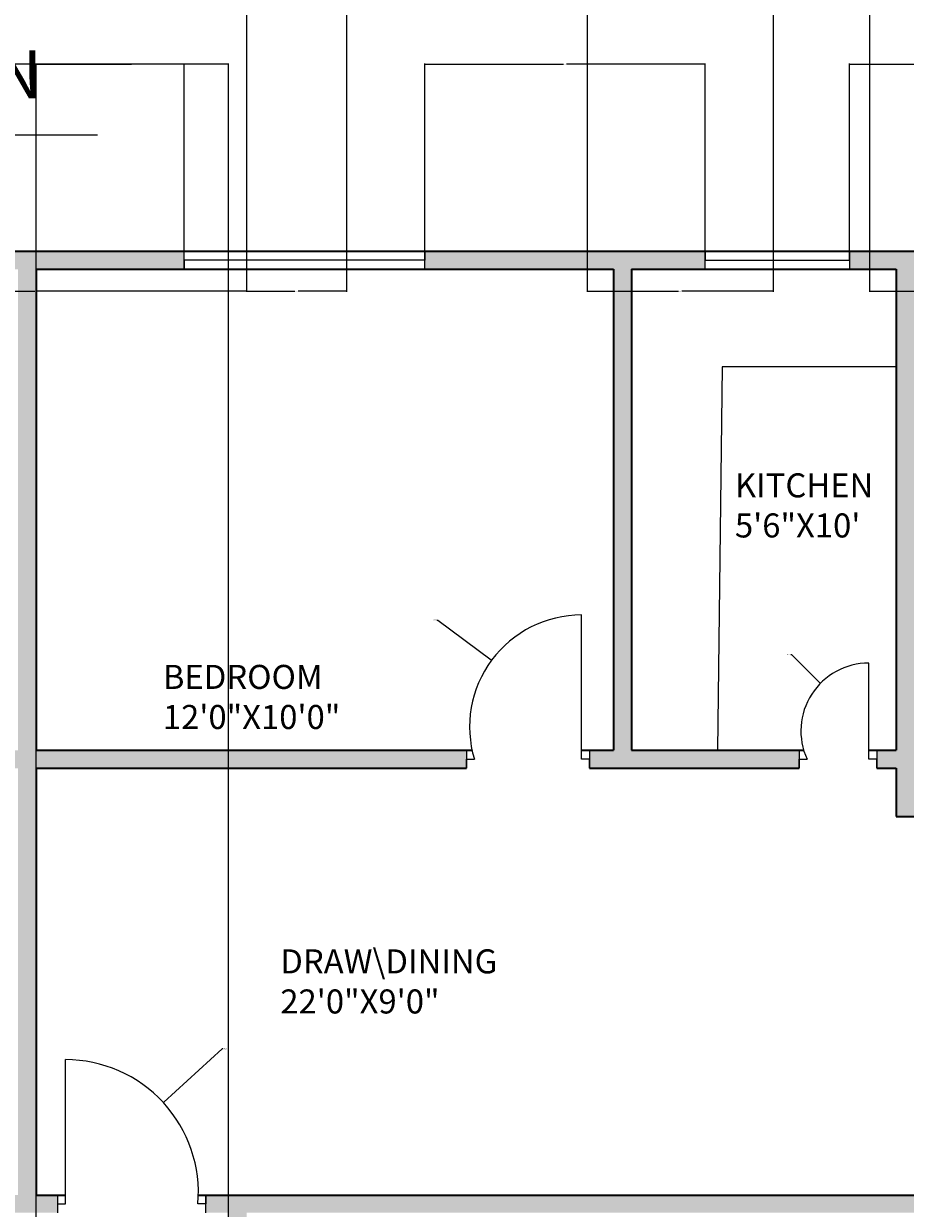
# Model space of a CAD drawing. Units: inches. Extents: x 2314 to 3223, y 1382 to 2735.
# Tile 12 of 14: x 2767 to 2987, y 2143 to 2439. Entities that reach past the tile are written whole.
import ezdxf

# ---------------------------------------------------------------- set-up
doc = ezdxf.new("R2010")
doc.units = ezdxf.units.IN
for name, color, linetype, lineweight in [('A-ANNO-DIMS', 2, 'Continuous', 18), ('A-ANNO-TEXT', 7, 'Continuous', 25), ('A-AREA-IDEN', 7, 'Continuous', 18), ('A-DOOR', 3, 'Continuous', 18), ('A-FLOR-FIXT', 8, 'Continuous', 18), ('A-GLAZ', 4, 'Continuous', 18), ('A-WALL', 7, 'Continuous', 35)]:
    doc.layers.add(name, color=color, linetype=linetype, lineweight=lineweight)
doc.layers.add('A-WALL-PATT', color=251, linetype='Continuous', lineweight=13, true_color=0x636466)
doc.styles.get("Standard").update_dxf_attribs({"font": 'arial.ttf'})
doc.dimstyles.get("Standard").update_dxf_attribs({"dimtxt": 0.18, "dimasz": 0.18, "dimexe": 0.18, "dimexo": 0.0625, "dimgap": 0.09, "dimtad": 0, "dimtih": 1, "dimtoh": 1, "dimdec": 4, "dimzin": 0, "dimdsep": 46, "dimtxsty": 'Standard', "dimcen": 0.09, "dimadec": 0, "dimazin": 0, "dimtfac": 1, "dimtdec": 4, "dimtofl": 0, "dimtmove": 0, "dimatfit": 3, "dimfxl": 1, "dimtolj": 1, "dimtzin": 0, "dimarcsym": 0})

# ---------------------------------------------------------------- blocks, each defined once
blk = doc.blocks.new('WIN-PLAN-60')
for p, q in [((0, 4.5), (0, 0)), ((60, 2.25), (60, 4.5)), ((60, 4.5), (60, 0)), ((0, 0), (0, 2.25)), ((0, 2.25), (60, 2.25))]:
    blk.add_line(p, q)
blk = doc.blocks.new('WIN-PLAN-36-ALT')
for p, q in [((0, 36), (4.5, 36)), ((4.5, 36), (2.25, 36)), ((2.25, 36), (2.25, 0)), ((4.5, 0), (0, 0)), ((2.25, 0), (4.5, 0))]:
    blk.add_line(p, q)
blk = doc.blocks.new('*D30')
at = {"layer": 'A-ANNO-DIMS', "color": 0, "lineweight": -2, "transparency": 16777216}
for p, q in [((3125.96, 2381.78), (3172.77, 2381.78)), ((3172.59, 2381.6), (3172.59, 1973.38)), ((3172.59, 1564.8), (3172.59, 1973.02)), ((2822.96, 1564.62), (3172.77, 1564.62))]:
    blk.add_line(p, q, dxfattribs=at)
at = {"layer": 'A-ANNO-DIMS', "color": 0, "transparency": 16777216}
for points in [[(3172.56, 2381.6), (3172.62, 2381.6), (3172.59, 2381.78)], [(3172.56, 1564.8), (3172.62, 1564.8), (3172.59, 1564.62)]]:
    blk.add_solid(points, dxfattribs=at)
at = {"layer": 'Defpoints', "color": 0, "transparency": 16777216}
for p in [(3125.89, 2381.78), (2822.89, 1564.62), (3172.59, 1564.62)]:
    blk.add_point(p, dxfattribs=at)
at = {"layer": 'A-ANNO-DIMS', "color": 0, "transparency": 16777216, "insert": (3172.59, 1973.2), "char_height": 0.18, "attachment_point": 5}
blk.add_mtext('\\A1;817.2', dxfattribs=at)
blk = doc.blocks.new('*D39')
at = {"layer": 'A-ANNO-DIMS', "color": 0, "lineweight": -2, "transparency": 16777216}
for p, q in [((2770.39, 1744.06), (2770.39, 2428.66)), ((2770.57, 2428.48), (2794.17, 2428.48)), ((2818.21, 2428.48), (2794.62, 2428.48)), ((2818.39, 1744.06), (2818.39, 2428.66))]:
    blk.add_line(p, q, dxfattribs=at)
at = {"layer": 'A-ANNO-DIMS', "color": 0, "transparency": 16777216}
for points in [[(2770.57, 2428.51), (2770.57, 2428.45), (2770.39, 2428.48)], [(2818.21, 2428.51), (2818.21, 2428.45), (2818.39, 2428.48)]]:
    blk.add_solid(points, dxfattribs=at)
at = {"layer": 'Defpoints', "color": 0, "transparency": 16777216}
for p in [(2818.39, 2428.48), (2770.39, 1744), (2818.39, 1744)]:
    blk.add_point(p, dxfattribs=at)
at = {"layer": 'A-ANNO-DIMS', "color": 0, "transparency": 16777216, "insert": (2794.39, 2428.48), "char_height": 0.18, "attachment_point": 5}
blk.add_mtext('\\A1;48', dxfattribs=at)
blk = doc.blocks.new('*D43')
at = {"layer": 'A-ANNO-DIMS', "color": 0, "lineweight": -2, "transparency": 16777216}
for p, q in [((2716.06, 2381.85), (2716.06, 2428.66)), ((2716.24, 2428.48), (2761.31, 2428.48)), ((2807.16, 2428.48), (2762.1, 2428.48)), ((2807.34, 2381.85), (2807.34, 2428.66))]:
    blk.add_line(p, q, dxfattribs=at)
at = {"layer": 'A-ANNO-DIMS', "color": 0, "transparency": 16777216}
for points in [[(2716.24, 2428.51), (2716.24, 2428.45), (2716.06, 2428.48)], [(2807.16, 2428.51), (2807.16, 2428.45), (2807.34, 2428.48)]]:
    blk.add_solid(points, dxfattribs=at)
at = {"layer": 'Defpoints', "color": 0, "transparency": 16777216}
for p in [(2807.34, 2428.48), (2716.06, 2381.78), (2807.34, 2381.78)]:
    blk.add_point(p, dxfattribs=at)
at = {"layer": 'A-ANNO-DIMS', "color": 0, "transparency": 16777216, "insert": (2761.7, 2428.48), "char_height": 0.18, "attachment_point": 5}
blk.add_mtext('\\A1;91.28', dxfattribs=at)
blk = doc.blocks.new('*D44')
at = {"layer": 'A-ANNO-DIMS', "color": 0, "lineweight": -2, "transparency": 16777216}
for p, q in [((2867.34, 2381.85), (2867.34, 2428.66)), ((2867.52, 2428.48), (2901.88, 2428.48)), ((2937.03, 2428.48), (2902.67, 2428.48)), ((2937.21, 2381.85), (2937.21, 2428.66))]:
    blk.add_line(p, q, dxfattribs=at)
at = {"layer": 'A-ANNO-DIMS', "color": 0, "transparency": 16777216}
for points in [[(2867.52, 2428.51), (2867.52, 2428.45), (2867.34, 2428.48)], [(2937.03, 2428.51), (2937.03, 2428.45), (2937.21, 2428.48)]]:
    blk.add_solid(points, dxfattribs=at)
at = {"layer": 'Defpoints', "color": 0, "transparency": 16777216}
for p in [(2937.21, 2428.48), (2867.34, 2381.78), (2937.21, 2381.78)]:
    blk.add_point(p, dxfattribs=at)
at = {"layer": 'A-ANNO-DIMS', "color": 0, "transparency": 16777216, "insert": (2902.28, 2428.48), "char_height": 0.18, "attachment_point": 5}
blk.add_mtext('\\A1;69.87', dxfattribs=at)
blk = doc.blocks.new('*D45')
at = {"layer": 'A-ANNO-DIMS', "color": 0, "lineweight": -2, "transparency": 16777216}
for p, q in [((2973.21, 2381.85), (2973.21, 2428.66)), ((2973.39, 2428.48), (2997.29, 2428.48)), ((3021.98, 2428.48), (2998.08, 2428.48)), ((3022.16, 2381.85), (3022.16, 2428.66))]:
    blk.add_line(p, q, dxfattribs=at)
at = {"layer": 'A-ANNO-DIMS', "color": 0, "transparency": 16777216}
for points in [[(2973.39, 2428.51), (2973.39, 2428.45), (2973.21, 2428.48)], [(3021.98, 2428.51), (3021.98, 2428.45), (3022.16, 2428.48)]]:
    blk.add_solid(points, dxfattribs=at)
at = {"layer": 'Defpoints', "color": 0, "transparency": 16777216}
for p in [(3022.16, 2428.48), (2973.21, 2381.78), (3022.16, 2381.78)]:
    blk.add_point(p, dxfattribs=at)
at = {"layer": 'A-ANNO-DIMS', "color": 0, "transparency": 16777216, "insert": (2997.69, 2428.48), "char_height": 0.18, "attachment_point": 5}
blk.add_mtext('\\A1;48.95', dxfattribs=at)
blk = doc.blocks.new('*D56')
at = {"layer": 'A-ANNO-DIMS', "color": 0, "lineweight": -2, "transparency": 16777216}
for p, q in [((2717.89, 2466.62), (2717.89, 2371.63)), ((2822.89, 2466.62), (2822.89, 2371.63)), ((2718.07, 2371.81), (2770.11, 2371.81)), ((2822.71, 2371.81), (2770.67, 2371.81))]:
    blk.add_line(p, q, dxfattribs=at)
at = {"layer": 'A-ANNO-DIMS', "color": 0, "transparency": 16777216}
for points in [[(2718.07, 2371.84), (2718.07, 2371.78), (2717.89, 2371.81)], [(2822.71, 2371.84), (2822.71, 2371.78), (2822.89, 2371.81)]]:
    blk.add_solid(points, dxfattribs=at)
at = {"layer": 'Defpoints', "color": 0, "transparency": 16777216}
for p in [(2717.89, 2466.68), (2822.89, 2466.68), (2822.89, 2371.81)]:
    blk.add_point(p, dxfattribs=at)
at = {"layer": 'A-ANNO-DIMS', "color": 0, "transparency": 16777216, "insert": (2770.39, 2371.81), "char_height": 0.18, "attachment_point": 5}
blk.add_mtext('\\A1;105', dxfattribs=at)
blk = doc.blocks.new('*D57')
at = {"layer": 'A-ANNO-DIMS', "color": 0, "lineweight": -2, "transparency": 16777216}
for p, q in [((2847.78, 2502.62), (2847.78, 2371.63)), ((2822.89, 2466.62), (2822.89, 2371.63)), ((2823.07, 2371.81), (2834.94, 2371.81)), ((2847.6, 2371.81), (2835.73, 2371.81))]:
    blk.add_line(p, q, dxfattribs=at)
at = {"layer": 'A-ANNO-DIMS', "color": 0, "transparency": 16777216}
for points in [[(2823.07, 2371.84), (2823.07, 2371.78), (2822.89, 2371.81)], [(2847.6, 2371.84), (2847.6, 2371.78), (2847.78, 2371.81)]]:
    blk.add_solid(points, dxfattribs=at)
at = {"layer": 'Defpoints', "color": 0, "transparency": 16777216}
for p in [(2847.78, 2502.68), (2822.89, 2466.68), (2847.78, 2371.81)]:
    blk.add_point(p, dxfattribs=at)
at = {"layer": 'A-ANNO-DIMS', "color": 0, "transparency": 16777216, "insert": (2835.34, 2371.81), "char_height": 0.18, "attachment_point": 5}
blk.add_mtext('\\A1;24.89', dxfattribs=at)
blk = doc.blocks.new('*D58')
at = {"layer": 'A-ANNO-DIMS', "color": 0, "lineweight": -2, "transparency": 16777216}
for p, q in [((2907.78, 2502.62), (2907.78, 2371.63)), ((2954.22, 2502.62), (2954.22, 2371.63)), ((2907.96, 2371.81), (2930.61, 2371.81)), ((2954.04, 2371.81), (2931.4, 2371.81))]:
    blk.add_line(p, q, dxfattribs=at)
at = {"layer": 'A-ANNO-DIMS', "color": 0, "transparency": 16777216}
for points in [[(2907.96, 2371.84), (2907.96, 2371.78), (2907.78, 2371.81)], [(2954.04, 2371.84), (2954.04, 2371.78), (2954.22, 2371.81)]]:
    blk.add_solid(points, dxfattribs=at)
at = {"layer": 'Defpoints', "color": 0, "transparency": 16777216}
for p in [(2907.78, 2502.68), (2954.22, 2502.68), (2954.22, 2371.81)]:
    blk.add_point(p, dxfattribs=at)
at = {"layer": 'A-ANNO-DIMS', "color": 0, "transparency": 16777216, "insert": (2931, 2371.81), "char_height": 0.18, "attachment_point": 5}
blk.add_mtext('\\A1;46.44', dxfattribs=at)
blk = doc.blocks.new('*D59')
at = {"layer": 'A-ANNO-DIMS', "color": 0, "lineweight": -2, "transparency": 16777216}
for p, q in [((2978.22, 2502.62), (2978.22, 2371.63)), ((3034.7, 2502.62), (3034.7, 2371.63)), ((2978.4, 2371.81), (3006.07, 2371.81)), ((3034.52, 2371.81), (3006.85, 2371.81))]:
    blk.add_line(p, q, dxfattribs=at)
at = {"layer": 'A-ANNO-DIMS', "color": 0, "transparency": 16777216}
for points in [[(2978.4, 2371.84), (2978.4, 2371.78), (2978.22, 2371.81)], [(3034.52, 2371.84), (3034.52, 2371.78), (3034.7, 2371.81)]]:
    blk.add_solid(points, dxfattribs=at)
at = {"layer": 'Defpoints', "color": 0, "transparency": 16777216}
for p in [(2978.22, 2502.68), (3034.7, 2502.68), (3034.7, 2371.81)]:
    blk.add_point(p, dxfattribs=at)
at = {"layer": 'A-ANNO-DIMS', "color": 0, "transparency": 16777216, "insert": (3006.46, 2371.81), "char_height": 0.18, "attachment_point": 5}
blk.add_mtext('\\A1;56.47', dxfattribs=at)
blk = doc.blocks.new('*D64')
at = {"layer": 'A-ANNO-DIMS', "color": 0, "lineweight": -2, "transparency": 16777216}
for p, q in [((2816.79, 2182.78), (2802.27, 2169.46)), ((2816.97, 2182.78), (2816.79, 2182.78)), ((2777.62, 2146.94), (2777.8, 2146.94)), ((2777.71, 2146.85), (2777.71, 2147.03))]:
    blk.add_line(p, q, dxfattribs=at)
at = {"layer": 'A-ANNO-DIMS', "color": 0, "transparency": 16777216}
blk.add_solid([(2802.25, 2169.49), (2802.29, 2169.44), (2802.14, 2169.34)], dxfattribs=at)
at = {"layer": 'Defpoints', "color": 0, "transparency": 16777216}
for p in [(2802.14, 2169.34), (2777.71, 2146.94)]:
    blk.add_point(p, dxfattribs=at)
at = {"layer": 'A-ANNO-DIMS', "color": 0, "transparency": 16777216, "insert": (2817.45, 2182.78), "char_height": 0.18, "attachment_point": 5}
blk.add_mtext('\\A1;R33.14', dxfattribs=at)
blk = doc.blocks.new('*D75')
at = {"layer": 'A-ANNO-DIMS', "color": 0, "lineweight": -2, "transparency": 16777216}
for p, q in [((2870.36, 2289.74), (2870.54, 2289.74)), ((2870.54, 2289.74), (2883.85, 2279.86)), ((2906.32, 2263.11), (2906.5, 2263.11)), ((2906.41, 2263.02), (2906.41, 2263.2))]:
    blk.add_line(p, q, dxfattribs=at)
at = {"layer": 'A-ANNO-DIMS', "color": 0, "transparency": 16777216}
blk.add_solid([(2883.87, 2279.89), (2883.83, 2279.84), (2883.99, 2279.76)], dxfattribs=at)
at = {"layer": 'Defpoints', "color": 0, "transparency": 16777216}
for p in [(2883.99, 2279.76), (2906.41, 2263.11)]:
    blk.add_point(p, dxfattribs=at)
at = {"layer": 'A-ANNO-DIMS', "color": 0, "transparency": 16777216, "insert": (2869.88, 2289.74), "char_height": 0.18, "attachment_point": 5}
blk.add_mtext('\\A1;R27.92', dxfattribs=at)
blk = doc.blocks.new('*D90')
at = {"layer": 'A-ANNO-DIMS', "color": 0, "lineweight": -2, "transparency": 16777216}
for p, q in [((2958.59, 2281.15), (2958.77, 2281.15)), ((2958.77, 2281.15), (2965.87, 2274.12)), ((2977.97, 2262.08), (2978.15, 2262.08)), ((2978.06, 2261.99), (2978.06, 2262.17))]:
    blk.add_line(p, q, dxfattribs=at)
at = {"layer": 'A-ANNO-DIMS', "color": 0, "transparency": 16777216}
blk.add_solid([(2965.9, 2274.15), (2965.85, 2274.1), (2966, 2274)], dxfattribs=at)
at = {"layer": 'Defpoints', "color": 0, "transparency": 16777216}
for p in [(2966, 2274), (2978.06, 2262.08)]:
    blk.add_point(p, dxfattribs=at)
at = {"layer": 'A-ANNO-DIMS', "color": 0, "transparency": 16777216, "insert": (2958.11, 2281.15), "char_height": 0.18, "attachment_point": 5}
blk.add_mtext('\\A1;R16.95', dxfattribs=at)

msp = doc.modelspace()

# ---------------------------------------------------------------- hatches: boundary and pattern name
at = {"layer": 'A-WALL-PATT'}
h = msp.add_hatch(color=256, dxfattribs=at)
h.dxf.hatch_style = 1
h.paths.add_polyline_path([(2443.3302, 2379.5332), (2443.3302, 2381.7832), (2410.3927, 2381.7832), (2410.3927, 2336.7008), (2414.8927, 2336.7008), (2414.8927, 2377.2832), (2443.3302, 2377.2832)])
h.paths.add_polyline_path([(2561.3645, 2379.5332), (2561.3645, 2381.7832), (2503.3302, 2381.7832), (2503.3302, 2377.2832), (2546.8927, 2377.2832), (2546.8927, 2245.2832), (2541.8787, 2245.2832), (2541.8787, 2240.7832), (2551.3927, 2240.7832), (2551.3927, 2377.2832), (2561.3645, 2377.2832)])
h.paths.add_polyline_path([(2656.0607, 2381.7832), (2597.3645, 2381.7832), (2597.3645, 2377.2832), (2617.3927, 2377.2832), (2617.3927, 2257.2832), (2584.2532, 2257.2832), (2584.2532, 2252.7832), (2625.8528, 2252.7832), (2625.8528, 2255.0332), (2625.8528, 2257.2832), (2621.8927, 2257.2832), (2621.8927, 2377.2832), (2656.0607, 2377.2832), (2656.0607, 2379.5332)])
h.paths.add_polyline_path([(2807.3418, 2381.7832), (2716.0607, 2381.7832), (2716.0607, 2377.2832), (2765.8927, 2377.2832), (2765.8927, 2257.2832), (2661.6935, 2257.2832), (2661.6935, 2252.7832), (2765.8927, 2252.7832), (2765.8927, 2146.2832), (2760.9259, 2146.2832), (2760.9259, 2141.8832), (2775.7119, 2141.8832), (2775.7119, 2146.2832), (2770.3927, 2146.2832), (2770.3927, 2252.7832), (2877.684, 2252.7832), (2877.684, 2255.0332), (2877.684, 2257.2832), (2770.3927, 2257.2832), (2770.3927, 2377.2832), (2807.3418, 2377.2832), (2807.3418, 2379.5332)])
h.paths.add_polyline_path([(2937.2118, 2381.7832), (2867.3418, 2381.7832), (2867.3418, 2377.2832), (2914.3927, 2377.2832), (2914.3927, 2257.2832), (2908.4124, 2257.2832), (2908.4124, 2252.7832), (2960.6432, 2252.7832), (2960.6432, 2255.0332), (2960.6432, 2257.2832), (2918.8927, 2257.2832), (2918.8927, 2377.2832), (2937.2118, 2377.2832)])
h.paths.add_polyline_path([(3022.1601, 2381.7832), (2973.2118, 2381.7832), (2973.2118, 2379.5332), (2973.2118, 2377.2832), (2984.8927, 2377.2832), (2984.8927, 2257.2832), (2980.0601, 2257.2832), (2980.0601, 2252.7832), (2984.8927, 2252.7832), (2984.8927, 2240.7832), (2995.668, 2240.7832), (2995.668, 2243.0332), (2995.668, 2245.2832), (2989.3927, 2245.2832), (2989.3927, 2377.2832), (3022.1601, 2377.2832), (3022.1601, 2379.5332)])
h.paths.add_polyline_path([(3125.8927, 2381.7832), (3082.1601, 2381.7832), (3082.1601, 2377.2832), (3121.3927, 2377.2832), (3121.3927, 2334.7388), (3125.8927, 2334.7388)])
h.paths.add_polyline_path([(3125.8927, 2274.7388), (3121.3927, 2274.7388), (3121.3927, 2245.2832), (3066.4832, 2245.2832), (3066.4832, 2240.7832), (3121.3927, 2240.7832), (3121.3927, 2232.1868), (3125.8927, 2232.1868)])
h.paths.add_polyline_path([(3125.8927, 2208.1868), (3121.3927, 2208.1868), (3121.3927, 2198.7832), (3037.3927, 2198.7832), (3037.3927, 2240.7832), (3041.2694, 2240.7832), (3041.2694, 2243.0332), (3041.2694, 2245.2832), (3026.8205, 2245.2832), (3026.8205, 2240.7832), (3032.8927, 2240.7832), (3032.8927, 2190.4022), (3037.3927, 2190.4022), (3037.3927, 2194.2832), (3121.3927, 2194.2832), (3121.3927, 2182.1835), (3125.8927, 2182.1835)])
h.paths.add_polyline_path([(3125.8927, 2158.1835), (3121.3927, 2158.1835), (3121.3927, 2146.2832), (3037.3927, 2146.2832), (3037.3927, 2169.3726), (3035.1427, 2169.3726), (3032.8927, 2169.3726), (3032.8927, 2146.2832), (2812.7301, 2146.2832), (2812.7301, 2144.0832), (2812.7301, 2141.8832), (2818.3927, 2141.8832), (2818.3927, 1970.1316), (2822.8927, 1970.1316), (2822.8927, 1978.8832), (2903.9846, 1978.8832), (2903.9846, 1981.1332), (2903.9846, 1983.3832), (2822.8927, 1983.3832), (2822.8927, 2115.3832), (2851.7162, 2115.3832), (2851.7162, 2117.6332), (2851.7162, 2119.8832), (2822.8927, 2119.8832), (2822.8927, 2141.8832), (3125.8927, 2141.8832)])
h.paths.add_polyline_path([(3125.8927, 2119.8832), (3081.193, 2119.8832), (3081.193, 2115.3832), (3121.3927, 2115.3832), (3121.3927, 2071.8188), (3125.8927, 2071.8188)], flags=17)
h.paths.add_polyline_path([(2989.3927, 2115.3832), (3021.193, 2115.3832), (3021.193, 2117.6332), (3021.193, 2119.8832), (2979.123, 2119.8832), (2979.123, 2115.3832), (2984.8927, 2115.3832), (2984.8927, 2019.3832), (2981.9225, 2019.3832), (2981.9225, 2014.8832), (2984.8927, 2014.8832), (2984.8927, 1983.3832), (2984.8927, 1978.8832), (2989.3927, 1978.8832), (2989.3927, 1983.3832)], flags=17)
h.paths.add_polyline_path([(2947.3927, 2115.3832), (2955.123, 2115.3832), (2955.123, 2117.6332), (2955.123, 2119.8832), (2911.7162, 2119.8832), (2911.7162, 2115.3832), (2942.8927, 2115.3832), (2942.8927, 1983.3832), (2936.7017, 1983.3832), (2936.7017, 1978.8832), (2947.3927, 1978.8832), (2947.3927, 1983.3832), (2947.3927, 2014.8832), (2960.7167, 2014.8832), (2960.7167, 2017.1332), (2960.7167, 2019.3832), (2947.3927, 2019.3832)], flags=17)
h.paths.add_polyline_path([(3037.3927, 1978.8832), (3041.8276, 1978.8832), (3041.8276, 1981.1332), (3041.8276, 1983.3832), (3025.477, 1983.3832), (3025.477, 1978.8832), (3032.8927, 1978.8832), (3032.8927, 1927.1259), (3035.1427, 1927.1259), (3037.3927, 1927.1259)])
h.paths.add_polyline_path([(3125.8927, 2011.8188), (3123.6427, 2011.8188), (3121.3927, 2011.8188), (3121.3927, 1983.3832), (3065, 1983.3832), (3065, 1978.8832), (3121.3927, 1978.8832), (3121.3927, 1970.5932), (3125.8927, 1970.5932)], flags=17)
h.paths.add_polyline_path([(2994.2341, 1983.3832), (2989.3927, 1983.3832), (2989.3927, 1978.8832), (2994.2341, 1978.8832), (2994.2341, 1981.1332)], flags=16)
h.paths.add_polyline_path([(3125.8927, 1946.5932), (3121.3927, 1946.5932), (3121.3927, 1936.8832), (3037.3927, 1936.8832), (3037.3927, 1932.3832), (3121.3927, 1932.3832), (3121.3927, 1919.825), (3125.8927, 1919.825)])
h.paths.add_polyline_path([(3125.8927, 1883.825), (3121.3927, 1883.825), (3121.3927, 1866.3832), (3037.3927, 1866.3832), (3037.3927, 1899.0954), (3035.1427, 1899.0954), (3032.8927, 1899.0954), (3032.8927, 1866.3832), (2822.8927, 1866.3832), (2822.8927, 1938.7212), (2820.6427, 1938.7212), (2818.3927, 1938.7212), (2818.3927, 1786.9239), (2822.8927, 1786.9239), (2822.8927, 1861.8832), (3032.8927, 1861.8832), (3032.8927, 1825.1023), (3037.3927, 1825.1023), (3037.3927, 1861.8832), (3121.3927, 1861.8832), (3121.3927, 1844.6765), (3125.8927, 1844.6765)])
h.paths.add_polyline_path([(3125.8927, 1808.6765), (3121.3927, 1808.6765), (3121.3927, 1795.8832), (3037.3927, 1795.8832), (3037.3927, 1799.4755), (3032.8927, 1799.4755), (3032.8927, 1749.3832), (3026.5034, 1749.3832), (3026.5034, 1744.8832), (3032.8927, 1744.8832), (3034.9255, 1744.8832), (3043.1326, 1744.8832), (3043.1326, 1747.1332), (3043.1326, 1749.3832), (3037.3927, 1749.3832), (3037.3927, 1791.3832), (3121.3927, 1791.3832), (3121.3927, 1783.3103), (3125.8927, 1783.3103)])
h.paths.add_polyline_path([(3125.8927, 1759.3103), (3121.3927, 1759.3103), (3121.3927, 1749.3832), (3065.1845, 1749.3832), (3065.1845, 1744.8832), (3121.3927, 1744.8832), (3121.3927, 1709.3573), (3125.8927, 1709.3573)])
h.paths.add_polyline_path([(3125.8927, 1649.3573), (3121.3927, 1649.3573), (3121.3927, 1612.8832), (3095.116, 1612.8832), (3095.116, 1608.3832), (3125.8927, 1608.3832)])
h.paths.add_polyline_path([(3035.116, 1612.8832), (2993.8927, 1612.8832), (2993.8927, 1744.8832), (2998.7409, 1744.8832), (2998.7409, 1749.3832), (2989.3927, 1749.3832), (2989.3927, 1744.8832), (2989.3927, 1701.3832), (2972.8226, 1701.3832), (2972.8226, 1696.8832), (2989.3927, 1696.8832), (2989.3927, 1612.8832), (2978.2225, 1612.8832), (2978.2225, 1608.3832), (3035.116, 1608.3832), (3035.116, 1610.6332)])
h.paths.add_polyline_path([(2947.3927, 1696.8832), (2950.7566, 1696.8832), (2950.7566, 1699.1332), (2950.7566, 1701.3832), (2947.3927, 1701.3832), (2947.3927, 1744.8832), (2947.3927, 1749.3832), (2937.649, 1749.3832), (2937.649, 1744.8832), (2942.8927, 1744.8832), (2942.8927, 1612.8832), (2907.783, 1612.8832), (2907.783, 1608.3832), (2954.2225, 1608.3832), (2954.2225, 1610.6332), (2954.2225, 1612.8832), (2947.3927, 1612.8832)])
h.paths.add_polyline_path([(2822.8927, 1744.8832), (2905.3491, 1744.8832), (2905.3491, 1747.1332), (2905.3491, 1749.3832), (2822.8927, 1749.3832), (2822.8927, 1756.9185), (2818.3927, 1756.9185), (2818.3927, 1612.8832), (2818.3927, 1569.1205), (2722.3927, 1569.1205), (2722.3927, 1612.8832), (2722.3927, 1756.9185), (2717.8927, 1756.9185), (2717.8927, 1750.0143), (2633.6297, 1750.0143), (2633.6437, 1745.2665), (2717.8927, 1745.5143), (2717.8927, 1612.8832), (2689.8467, 1612.8832), (2689.8467, 1608.3832), (2717.8927, 1608.3832), (2717.8927, 1564.6205), (2722.3927, 1564.6205), (2822.8927, 1564.6205), (2822.8927, 1569.1205), (2822.8927, 1608.3832), (2847.783, 1608.3832), (2847.783, 1610.6332), (2847.783, 1612.8832), (2822.8927, 1612.8832)])
h.paths.add_polyline_path([(2629.8467, 1612.8832), (2597.8927, 1612.8832), (2597.8927, 1744.8832), (2597.8927, 1745.1613), (2601.5887, 1745.1721), (2601.5816, 1747.5932), (2601.5745, 1750.0143), (2593.3927, 1750.0143), (2593.3927, 1744.8832), (2593.3927, 1713.3832), (2589.7588, 1713.3832), (2589.7588, 1708.8832), (2593.3927, 1708.8832), (2593.3927, 1612.8832), (2582.3793, 1612.8832), (2582.3793, 1608.3832), (2629.8467, 1608.3832), (2629.8467, 1610.6332)])
h.paths.add_polyline_path([(2551.3927, 1708.8832), (2567.6776, 1708.8832), (2567.6776, 1711.1332), (2567.6776, 1713.3832), (2551.3927, 1713.3832), (2551.3927, 1744.8832), (2551.3927, 1750.0143), (2543.5657, 1750.0143), (2543.5657, 1747.5079), (2543.5657, 1745.0014), (2546.8927, 1745.0112), (2546.8927, 1744.8832), (2546.8927, 1612.8832), (2502.9339, 1612.8832), (2502.9339, 1608.3832), (2558.3793, 1608.3832), (2558.3793, 1610.6332), (2558.3793, 1612.8832), (2551.3927, 1612.8832)])
h.paths.add_polyline_path([(2414.8927, 1656.2547), (2410.3927, 1656.2547), (2410.3927, 1608.3832), (2442.9339, 1608.3832), (2442.9339, 1610.6332), (2442.9339, 1612.8832), (2414.8927, 1612.8832)])
h.paths.add_polyline_path([(2414.8927, 1744.8832), (2468.8906, 1744.8832), (2468.8906, 1747.1332), (2468.8906, 1749.3832), (2414.8927, 1749.3832), (2414.8927, 1757.7622), (2410.3927, 1757.7622), (2410.3927, 1716.2547), (2414.8927, 1716.2547)])
h.paths.add_polyline_path([(2414.8927, 1791.3832), (2498.8927, 1791.3832), (2498.8927, 1749.3832), (2492.9799, 1749.3832), (2492.9799, 1744.8832), (2498.8927, 1744.8832), (2503.3927, 1744.8832), (2508.0135, 1744.8968), (2508.0059, 1747.4556), (2507.9984, 1750.0143), (2503.3927, 1750.0143), (2503.3927, 1802.6362), (2501.1427, 1802.6362), (2498.8927, 1802.6362), (2498.8927, 1795.8832), (2414.8927, 1795.8832), (2414.8927, 1808.0943), (2410.3927, 1808.0943), (2410.3927, 1781.7622), (2414.8927, 1781.7622)])
h.paths.add_polyline_path([(2722.3927, 1937.589), (2720.1427, 1937.589), (2717.8927, 1937.589), (2717.8927, 1866.3832), (2503.3927, 1866.3832), (2503.3927, 1896.3484), (2498.8927, 1896.3484), (2498.8927, 1866.3832), (2414.8927, 1866.3832), (2414.8927, 1882.1496), (2410.3927, 1882.1496), (2410.3927, 1844.0943), (2414.8927, 1844.0943), (2414.8927, 1861.8832), (2498.8927, 1861.8832), (2498.8927, 1831.4783), (2501.1427, 1831.4783), (2503.3927, 1831.4783), (2503.3927, 1861.8832), (2717.8927, 1861.8832), (2717.8927, 1786.9239), (2722.3927, 1786.9239)])
h.paths.add_polyline_path([(2414.8927, 1932.3832), (2498.8927, 1932.3832), (2498.8927, 1924.7883), (2503.3927, 1924.7883), (2503.3927, 1978.8832), (2505.8599, 1978.8832), (2505.8599, 1981.1332), (2505.8599, 1983.3832), (2493.3697, 1983.3832), (2493.3697, 1978.8832), (2498.8927, 1978.8832), (2498.8927, 1936.8832), (2414.8927, 1936.8832), (2414.8927, 1943.2834), (2410.3927, 1943.2834), (2410.3927, 1918.1496), (2414.8927, 1918.1496)])
h.paths.add_polyline_path([(2414.8927, 2020.3133), (2412.6427, 2020.3133), (2410.3927, 2020.3133), (2410.3927, 1967.2834), (2414.8927, 1967.2834), (2414.8927, 1978.8832), (2468.8513, 1978.8832), (2468.8513, 1981.1332), (2468.8513, 1983.3832), (2414.8927, 1983.3832)])
h.paths.add_polyline_path([(2414.8927, 2115.3832), (2453.004, 2115.3832), (2453.004, 2117.6332), (2453.004, 2119.8832), (2410.3927, 2119.8832), (2410.3927, 2080.3133), (2414.8927, 2080.3133)], flags=17)
h.paths.add_polyline_path([(2559.0969, 2117.6332), (2559.0969, 2119.8832), (2513.004, 2119.8832), (2513.004, 2115.3832), (2546.8927, 2115.3832), (2546.8927, 1983.3832), (2542.7531, 1983.3832), (2542.7531, 1978.8832), (2551.3927, 1978.8832), (2551.3927, 2014.8832), (2570.3098, 2014.8832), (2570.3098, 2017.1332), (2570.3098, 2019.3832), (2551.3927, 2019.3832), (2551.3927, 2115.3832), (2559.0969, 2115.3832)], flags=17)
h.paths.add_polyline_path([(2628.5073, 2117.6332), (2628.5073, 2119.8832), (2583.0969, 2119.8832), (2583.0969, 2115.3832), (2593.3927, 2115.3832), (2593.3927, 2019.3832), (2590.2108, 2019.3832), (2590.2108, 2014.8832), (2593.3927, 2014.8832), (2593.3927, 1978.8832), (2601.5907, 1978.8832), (2601.5907, 1981.1332), (2601.5907, 1983.3832), (2597.8927, 1983.3832), (2597.8927, 2115.3832), (2628.5073, 2115.3832)], flags=17)
h.paths.add_polyline_path([(2722.3927, 2141.8832), (2726.9871, 2141.8832), (2726.9871, 2144.2705), (2726.9871, 2146.2832), (2503.3927, 2146.2832), (2503.3927, 2168.2161), (2501.1427, 2168.2161), (2498.8927, 2168.2161), (2498.8927, 2146.2832), (2414.8927, 2146.2832), (2414.8927, 2156.5041), (2410.3927, 2156.5041), (2410.3927, 2141.8832), (2717.8927, 2141.8832), (2717.8927, 2119.8832), (2688.5073, 2119.8832), (2688.5073, 2115.3832), (2717.8927, 2115.3832), (2717.8927, 1983.3832), (2633.2454, 1983.3832), (2633.2454, 1978.8832), (2717.8927, 1978.8832), (2717.8927, 1970.1316), (2720.1427, 1970.1316), (2722.3927, 1970.1316)])
h.paths.add_polyline_path([(2557.3704, 1462.9278), (2940.0934, 1462.9278), (2940.0934, 1512.3848), (2557.3704, 1512.3848)], flags=9)
h.paths.add_polyline_path([(2846.2527, 1703.1384), (2892.8612, 1703.1384), (2892.8612, 1725.5272), (2846.2527, 1725.5272)], flags=25)
h.paths.add_polyline_path([(2885.6102, 1812.1147), (2946.1505, 1812.1147), (2946.1505, 1834.5035), (2885.6102, 1834.5035)], flags=25)
h.paths.add_polyline_path([(2885.6102, 1884.183), (2946.1505, 1884.183), (2946.1505, 1906.5718), (2885.6102, 1906.5718)], flags=25)
h.paths.add_polyline_path([(3066.365, 1705.5431), (3112.9735, 1705.5431), (3112.9735, 1727.9319), (3066.365, 1727.9319)], flags=9)
h.paths.add_polyline_path([(3061.8255, 1887.7513), (3101.6154, 1887.7513), (3101.6154, 1910.1401), (3061.8255, 1910.1401)], flags=25)
h.paths.add_polyline_path([(3063.3679, 1816.2121), (3103.1578, 1816.2121), (3103.1578, 1838.6009), (3063.3679, 1838.6009)], flags=25)
h.paths.add_polyline_path([(3053.3743, 1768.416), (3107.1329, 1768.416), (3107.1329, 1790.8048), (3053.3743, 1790.8048)], flags=25)
h.paths.add_polyline_path([(3061.6068, 1943.822), (3115.3653, 1943.822), (3115.3653, 1966.2109), (3061.6068, 1966.2109)], flags=9)
h.paths.add_polyline_path([(2745.0978, 1763.6604), (2797.9354, 1763.6604), (2797.9354, 1776.0247), (2745.0978, 1776.0247)], flags=9)
h.paths.add_polyline_path([(2574.2135, 1819.2586), (2634.7538, 1819.2586), (2634.7538, 1841.6474), (2574.2135, 1841.6474)], flags=25)
h.paths.add_polyline_path([(2574.2135, 1891.3269), (2634.7538, 1891.3269), (2634.7538, 1913.7157), (2574.2135, 1913.7157)], flags=25)
h.paths.add_polyline_path([(2638.4466, 1702.43), (2685.0551, 1702.43), (2685.0551, 1724.8188), (2638.4466, 1724.8188)], flags=25)
h.paths.add_polyline_path([(2435.9715, 1697.1215), (2482.5799, 1697.1215), (2482.5799, 1719.5103), (2435.9715, 1719.5103)], flags=9)
h.paths.add_polyline_path([(2431.2046, 1893.7833), (2470.9945, 1893.7833), (2470.9945, 1916.1721), (2431.2046, 1916.1721)], flags=25)
h.paths.add_polyline_path([(2439.8144, 1817.2116), (2479.6043, 1817.2116), (2479.6043, 1839.6004), (2439.8144, 1839.6004)], flags=25)
h.paths.add_polyline_path([(2441.2607, 1753.0942), (2495.0192, 1753.0942), (2495.0192, 1775.483), (2441.2607, 1775.483)], flags=25)
h.paths.add_polyline_path([(2421.216, 1945.3109), (2474.9746, 1945.3109), (2474.9746, 1967.6997), (2421.216, 1967.6997)], flags=25)
h.paths.add_polyline_path([(2585.4464, 1627.5703), (2585.4464, 1679), (2563.0576, 1679), (2563.0576, 1627.5703)], flags=9)
h.paths.add_polyline_path([(2978.3497, 1618.7039), (2978.3497, 1670.1337), (2955.9609, 1670.1337), (2955.9609, 1618.7039)], flags=9)
h.paths.add_polyline_path([(2975.9502, 2041.7828), (2975.9502, 2093.2125), (2953.5614, 2093.2125), (2953.5614, 2041.7828)], flags=25)
h.paths.add_polyline_path([(2835.6537, 1989.2068), (2882.2621, 1989.2068), (2882.2621, 2011.5956), (2835.6537, 2011.5956)], flags=25)
h.paths.add_polyline_path([(2649.3769, 1997.5659), (2695.9853, 1997.5659), (2695.9853, 2019.9547), (2649.3769, 2019.9547)], flags=25)
h.paths.add_polyline_path([(2579.9087, 2040.3429), (2579.9087, 2091.7726), (2557.5198, 2091.7726), (2557.5198, 2040.3429)], flags=25)
h.paths.add_polyline_path([(2783.2404, 1883.1956), (2783.2404, 2067.1369), (2764.694, 2067.1369), (2764.694, 1883.1956)], flags=9)
h.paths.add_polyline_path([(3055.8435, 1993.5571), (3102.4519, 1993.5571), (3102.4519, 2015.9459), (3055.8435, 2015.9459)], flags=25)
h.paths.add_polyline_path([(2423.6009, 1984.6082), (2470.2094, 1984.6082), (2470.2094, 2006.997), (2423.6009, 2006.997)], flags=25)
h.paths.add_polyline_path([(2973.4115, 2123.1668), (3013.1319, 2123.1668), (3013.1319, 2135.531), (2973.4115, 2135.531)], flags=25)
h.paths.add_polyline_path([(2534.3846, 2124.6231), (2574.105, 2124.6231), (2574.105, 2136.9874), (2534.3846, 2136.9874)], flags=25)
h.paths.add_polyline_path([(2829.1368, 2188.1931), (2889.411, 2188.1931), (2889.411, 2210.5819), (2829.1368, 2210.5819)], flags=9)
h.paths.add_polyline_path([(2633.2547, 2185.0437), (2693.5289, 2185.0437), (2693.5289, 2207.4325), (2633.2547, 2207.4325)], flags=9)
h.paths.add_polyline_path([(2445.1812, 2167.0395), (2496.611, 2167.0395), (2496.611, 2189.4284), (2445.1812, 2189.4284)], flags=9)
h.paths.add_polyline_path([(2429.1678, 2194.5482), (2480.5975, 2194.5482), (2480.5975, 2216.937), (2429.1678, 2216.937)], flags=9)
h.paths.add_polyline_path([(3060.1138, 2158.1056), (3111.5436, 2158.1056), (3111.5436, 2180.4944), (3060.1138, 2180.4944)], flags=9)
h.paths.add_polyline_path([(3055.6824, 2201.2631), (3107.1122, 2201.2631), (3107.1122, 2223.652), (3055.6824, 2223.652)], flags=25)
h.paths.add_polyline_path([(3044.3482, 2257.7345), (3090.9567, 2257.7345), (3090.9567, 2280.1233), (3044.3482, 2280.1233)], flags=9)
h.paths.add_polyline_path([(2942.5437, 2306.9625), (2982.3336, 2306.9625), (2982.3336, 2329.3513), (2942.5437, 2329.3513)], flags=9)
h.paths.add_polyline_path([(2799.5865, 2259.1663), (2846.195, 2259.1663), (2846.195, 2281.5551), (2799.5865, 2281.5551)], flags=25)
h.paths.add_polyline_path([(2670.4998, 2261.1493), (2717.1082, 2261.1493), (2717.1082, 2283.5381), (2670.4998, 2283.5381)], flags=25)
h.paths.add_polyline_path([(2553.0333, 2302.7735), (2592.8232, 2302.7735), (2592.8232, 2325.1624), (2553.0333, 2325.1624)], flags=9)
h.paths.add_polyline_path([(2432.0288, 2268.6489), (2478.6372, 2268.6489), (2478.6372, 2291.0377), (2432.0288, 2291.0377)], flags=9)
h = msp.add_hatch(color=256, dxfattribs=at)
h.dxf.hatch_style = 1
h.paths.add_polyline_path([(2503.3927, 2240.7832), (2507.7952, 2240.7832), (2507.7952, 2245.2832), (2496.4262, 2245.2832), (2496.4262, 2243.0332), (2496.4262, 2240.7832), (2498.8927, 2240.7832), (2498.8927, 2198.7832), (2414.8927, 2198.7832), (2414.8927, 2206.5718), (2410.3927, 2206.5718), (2410.3927, 2180.5041), (2412.6427, 2180.5041), (2414.8927, 2180.5041), (2414.8927, 2194.2832), (2498.8927, 2194.2832), (2498.8927, 2191.0069), (2503.3927, 2191.0069)])
h.paths.add_polyline_path([(2414.8927, 2276.7008), (2410.3927, 2276.7008), (2410.3927, 2230.5718), (2414.8927, 2230.5718), (2414.8927, 2240.7832), (2474.2564, 2240.7832), (2474.2564, 2243.0332), (2474.2564, 2245.2832), (2414.8927, 2245.2832)])
h.paths.add_polyline_path([(2557.3704, 1462.9278), (2940.0934, 1462.9278), (2940.0934, 1512.3848), (2557.3704, 1512.3848)], flags=9)
h.paths.add_polyline_path([(2846.2527, 1703.1384), (2892.8612, 1703.1384), (2892.8612, 1725.5272), (2846.2527, 1725.5272)], flags=9)
h.paths.add_polyline_path([(2885.6102, 1812.1147), (2946.1505, 1812.1147), (2946.1505, 1834.5035), (2885.6102, 1834.5035)], flags=9)
h.paths.add_polyline_path([(2885.6102, 1884.183), (2946.1505, 1884.183), (2946.1505, 1906.5718), (2885.6102, 1906.5718)], flags=9)
h.paths.add_polyline_path([(3066.365, 1705.5431), (3112.9735, 1705.5431), (3112.9735, 1727.9319), (3066.365, 1727.9319)], flags=9)
h.paths.add_polyline_path([(3061.8255, 1887.7513), (3101.6154, 1887.7513), (3101.6154, 1910.1401), (3061.8255, 1910.1401)], flags=9)
h.paths.add_polyline_path([(3063.3679, 1816.2121), (3103.1578, 1816.2121), (3103.1578, 1838.6009), (3063.3679, 1838.6009)], flags=9)
h.paths.add_polyline_path([(3053.3743, 1768.416), (3107.1329, 1768.416), (3107.1329, 1790.8048), (3053.3743, 1790.8048)], flags=9)
h.paths.add_polyline_path([(3061.6068, 1943.822), (3115.3653, 1943.822), (3115.3653, 1966.2109), (3061.6068, 1966.2109)], flags=9)
h.paths.add_polyline_path([(2745.0978, 1763.6604), (2797.9354, 1763.6604), (2797.9354, 1776.0247), (2745.0978, 1776.0247)], flags=9)
h.paths.add_polyline_path([(2574.2135, 1819.2586), (2634.7538, 1819.2586), (2634.7538, 1841.6474), (2574.2135, 1841.6474)], flags=9)
h.paths.add_polyline_path([(2574.2135, 1891.3269), (2634.7538, 1891.3269), (2634.7538, 1913.7157), (2574.2135, 1913.7157)], flags=9)
h.paths.add_polyline_path([(2638.4466, 1702.43), (2685.0551, 1702.43), (2685.0551, 1724.8188), (2638.4466, 1724.8188)], flags=9)
h.paths.add_polyline_path([(2435.9715, 1697.1215), (2482.5799, 1697.1215), (2482.5799, 1719.5103), (2435.9715, 1719.5103)], flags=9)
h.paths.add_polyline_path([(2431.2046, 1893.7833), (2470.9945, 1893.7833), (2470.9945, 1916.1721), (2431.2046, 1916.1721)], flags=9)
h.paths.add_polyline_path([(2439.8144, 1817.2116), (2479.6043, 1817.2116), (2479.6043, 1839.6004), (2439.8144, 1839.6004)], flags=9)
h.paths.add_polyline_path([(2441.2607, 1753.0942), (2495.0192, 1753.0942), (2495.0192, 1775.483), (2441.2607, 1775.483)], flags=9)
h.paths.add_polyline_path([(2421.216, 1945.3109), (2474.9746, 1945.3109), (2474.9746, 1967.6997), (2421.216, 1967.6997)], flags=9)
h.paths.add_polyline_path([(2585.4464, 1627.5703), (2585.4464, 1679), (2563.0576, 1679), (2563.0576, 1627.5703)], flags=9)
h.paths.add_polyline_path([(2978.3497, 1618.7039), (2978.3497, 1670.1337), (2955.9609, 1670.1337), (2955.9609, 1618.7039)], flags=9)
h.paths.add_polyline_path([(2975.9502, 2041.7828), (2975.9502, 2093.2125), (2953.5614, 2093.2125), (2953.5614, 2041.7828)], flags=9)
h.paths.add_polyline_path([(2835.6537, 1989.2068), (2882.2621, 1989.2068), (2882.2621, 2011.5956), (2835.6537, 2011.5956)], flags=9)
h.paths.add_polyline_path([(2649.3769, 1997.5659), (2695.9853, 1997.5659), (2695.9853, 2019.9547), (2649.3769, 2019.9547)], flags=9)
h.paths.add_polyline_path([(2579.9087, 2040.3429), (2579.9087, 2091.7726), (2557.5198, 2091.7726), (2557.5198, 2040.3429)], flags=9)
h.paths.add_polyline_path([(2783.2404, 1883.1956), (2783.2404, 2067.1369), (2764.694, 2067.1369), (2764.694, 1883.1956)], flags=9)
h.paths.add_polyline_path([(3055.8435, 1993.5571), (3102.4519, 1993.5571), (3102.4519, 2015.9459), (3055.8435, 2015.9459)], flags=9)
h.paths.add_polyline_path([(2423.6009, 1984.6082), (2470.2094, 1984.6082), (2470.2094, 2006.997), (2423.6009, 2006.997)], flags=9)
h.paths.add_polyline_path([(2973.4115, 2123.1668), (3013.1319, 2123.1668), (3013.1319, 2135.531), (2973.4115, 2135.531)], flags=9)
h.paths.add_polyline_path([(2534.3846, 2124.6231), (2574.105, 2124.6231), (2574.105, 2136.9874), (2534.3846, 2136.9874)], flags=9)
h.paths.add_polyline_path([(2829.1368, 2188.1931), (2889.411, 2188.1931), (2889.411, 2210.5819), (2829.1368, 2210.5819)], flags=9)
h.paths.add_polyline_path([(2633.2547, 2185.0437), (2693.5289, 2185.0437), (2693.5289, 2207.4325), (2633.2547, 2207.4325)], flags=9)
h.paths.add_polyline_path([(2445.1812, 2167.0395), (2496.611, 2167.0395), (2496.611, 2189.4284), (2445.1812, 2189.4284)], flags=9)
h.paths.add_polyline_path([(2429.1678, 2208.3022), (2480.5975, 2208.3022), (2480.5975, 2230.691), (2429.1678, 2230.691)], flags=25)
h.paths.add_polyline_path([(3060.1138, 2158.1056), (3111.5436, 2158.1056), (3111.5436, 2180.4944), (3060.1138, 2180.4944)], flags=9)
h.paths.add_polyline_path([(3055.6824, 2201.2631), (3107.1122, 2201.2631), (3107.1122, 2223.652), (3055.6824, 2223.652)], flags=9)
h.paths.add_polyline_path([(3044.3482, 2257.7345), (3090.9567, 2257.7345), (3090.9567, 2280.1233), (3044.3482, 2280.1233)], flags=9)
h.paths.add_polyline_path([(2942.5437, 2306.9625), (2982.3336, 2306.9625), (2982.3336, 2329.3513), (2942.5437, 2329.3513)], flags=9)
h.paths.add_polyline_path([(2799.5865, 2259.1663), (2846.195, 2259.1663), (2846.195, 2281.5551), (2799.5865, 2281.5551)], flags=9)
h.paths.add_polyline_path([(2670.4998, 2261.1493), (2717.1082, 2261.1493), (2717.1082, 2283.5381), (2670.4998, 2283.5381)], flags=9)
h.paths.add_polyline_path([(2553.0333, 2302.7735), (2592.8232, 2302.7735), (2592.8232, 2325.1624), (2553.0333, 2325.1624)], flags=9)
h.paths.add_polyline_path([(2432.0288, 2268.6489), (2478.6372, 2268.6489), (2478.6372, 2291.0377), (2432.0288, 2291.0377)], flags=9)

# ---------------------------------------------------------------- linework, layer by layer
at = {"layer": 'A-ANNO-TEXT'}
msp.add_line((2675.75, 2410.8121), (2785.7373, 2410.8121), dxfattribs=at)
at = {"layer": 'A-DOOR'}
for p, q in [((2906.4124, 2255.0332), (2906.4124, 2291.0332)), ((2978.0601, 2255.0332), (2978.0601, 2279.0332)), ((2877.684, 2257.2832), (2877.684, 2252.7832)), ((2908.4124, 2257.2832), (2908.4124, 2252.7832)), ((2960.6432, 2257.2832), (2960.6432, 2252.7832)), ((2980.0601, 2257.2832), (2980.0601, 2252.7832)), ((2877.684, 2252.7832), (2877.684, 2255.0332)), ((2877.684, 2255.0332), (2879.684, 2255.0332)), ((2908.4124, 2255.0332), (2906.4124, 2255.0332)), ((2908.4124, 2252.7832), (2908.4124, 2255.0332)), ((2960.6432, 2252.7832), (2960.6432, 2255.0332)), ((2960.6432, 2255.0332), (2962.6432, 2255.0332)), ((2980.0601, 2255.0332), (2978.0601, 2255.0332)), ((2980.0601, 2252.7832), (2980.0601, 2255.0332)), ((2777.7119, 2144.0832), (2777.7119, 2180.0832)), ((2775.7119, 2146.2832), (2775.7119, 2141.8832)), ((2812.7301, 2141.8832), (2812.7301, 2146.2832)), ((2812.7301, 2146.2832), (2812.7301, 2144.0832)), ((2775.7119, 2144.0832), (2777.7119, 2144.0832)), ((2812.7301, 2144.0832), (2810.7301, 2144.0832))]:
    msp.add_line(p, q, dxfattribs=at)
for centre, radius, start, end in [((2906.4124, 2263.1109), 27.9224, 90, 196.815426), ((2978.0601, 2262.0816), 16.9517, 90, 204.569013), ((2777.7119, 2146.9416), 33.1417, 355.052322, 90)]:
    msp.add_arc(centre, radius, start, end, dxfattribs=at)
at = {"layer": 'A-FLOR-FIXT'}
for p, q in [((2941.451, 2352.9208), (2940.3472, 2257.2832)), ((2984.8927, 2352.9208), (2941.451, 2352.9208))]:
    msp.add_line(p, q, dxfattribs=at)
at = {"layer": 'A-WALL'}
for p, q in [((2410.3927, 2381.7832), (3125.8927, 2381.7832)), ((2770.3927, 2377.2832), (2770.3927, 2257.2832)), ((2770.3927, 2377.2832), (2914.3927, 2377.2832)), ((2914.3927, 2377.2832), (2914.3927, 2257.2832)), ((2918.8927, 2377.2832), (2918.8927, 2257.2832)), ((2918.8927, 2377.2832), (2984.8927, 2377.2832)), ((2984.8927, 2377.2832), (2984.8927, 2257.2832)), ((2770.3927, 2257.2832), (2879.105, 2257.2832)), ((2906.4124, 2257.2832), (2914.3927, 2257.2832)), ((2918.8927, 2257.2832), (2961.8017, 2257.2832)), ((2978.0601, 2257.2832), (2984.8927, 2257.2832)), ((2770.3927, 2252.7832), (2877.684, 2252.7832)), ((2770.3927, 2252.7832), (2770.3927, 2146.2832)), ((2908.4124, 2252.7832), (2960.6432, 2252.7832)), ((2980.0601, 2252.7832), (2984.8927, 2252.7832)), ((2984.8927, 2252.7832), (2984.8927, 2240.7832)), ((2984.8927, 2240.7832), (2995.668, 2240.7832)), ((2770.3927, 2146.2832), (2777.7119, 2146.2832)), ((2810.847, 2146.2832), (3032.8927, 2146.2832))]:
    msp.add_line(p, q, dxfattribs=at)

# ---------------------------------------------------------------- block references
at = {"layer": 'A-GLAZ'}
for name, p, rotation in [('WIN-PLAN-60', (2867.3418, 2381.7832), 180), ('WIN-PLAN-36-ALT', (2973.2118, 2377.2832), 89.9999999999985)]:
    msp.add_blockref(name, p, dxfattribs=dict(at, rotation=rotation))

# ---------------------------------------------------------------- texts
at = {"layer": 'A-ANNO-TEXT', "insert": (2685.687, 2431.9165), "char_height": 12, "attachment_point": 1}
msp.add_mtext_dynamic_manual_height_columns('ELEVATION', width=331.233746, gutter_width=12.5, heights=[0], dxfattribs=at)
at = {"layer": 'A-AREA-IDEN', "char_height": 6, "attachment_point": 1}
for s, width, insert in [('KITCHEN\\P5\'6"X10\'', 91.281907, (2944.6576, 2326.3656)), ('BEDROOM\\P12\'0"X10\'0"', 89.719354, (2801.9992, 2278.5735)), ('DRAW\\\\DINING\\P22\'0"X9\'0"', 93.899013, (2831.2835, 2207.5962))]:
    msp.add_mtext_dynamic_manual_height_columns(s, width=width, gutter_width=12.5, heights=[0], dxfattribs=dict(at, insert=insert))

# ---------------------------------------------------------------- dimensions: what is measured, and where the dimension line sits
at = {"layer": 'A-ANNO-DIMS'}
for base, p1, p2, override, picture, middle in [((2847.783, 2371.8121), (2822.8927, 2466.6793), (2847.783, 2502.6793), {"dimdec": 2, "dimlfac": 1, "dimrnd": 0, "dimzin": 0, "dimdsep": 46, "dimlunit": 2}, '*D57', (2835.3378, 2371.8121)), ((2954.2225, 2371.8121), (2907.783, 2502.6793), (2954.2225, 2502.6793), {"dimdec": 2, "dimlfac": 1, "dimrnd": 0, "dimzin": 0, "dimdsep": 46, "dimlunit": 2}, '*D58', (2931.0028, 2371.8121)), ((3034.6958, 2371.8121), (2978.2225, 2502.6793), (3034.6958, 2502.6793), {"dimdec": 2, "dimlfac": 1, "dimrnd": 0, "dimzin": 0, "dimdsep": 46, "dimlunit": 2}, '*D59', (3006.4592, 2371.8121)), ((2822.8927, 2371.8121), (2717.8927, 2466.6793), (2822.8927, 2466.6793), {"dimdec": 0, "dimlfac": 1, "dimrnd": 0, "dimzin": 0, "dimdsep": 46, "dimlunit": 2}, '*D56', (2770.3927, 2371.8121)), ((2807.3418, 2428.4832), (2716.0607, 2381.7832), (2807.3418, 2381.7832), {"dimdec": 2, "dimlfac": 1, "dimrnd": 0, "dimzin": 0, "dimdsep": 46, "dimlunit": 2}, '*D43', (2761.7012, 2428.4832)), ((2818.3927, 2428.4832), (2770.3927, 1743.998), (2818.3927, 1743.998), {"dimdec": 0, "dimlfac": 1, "dimrnd": 0, "dimzin": 0, "dimdsep": 46, "dimlunit": 2}, '*D39', (2794.3927, 2428.4832)), ((2937.2118, 2428.4832), (2867.3418, 2381.7832), (2937.2118, 2381.7832), {"dimdec": 2, "dimlfac": 1, "dimrnd": 0, "dimzin": 0, "dimdsep": 46, "dimlunit": 2}, '*D44', (2902.2768, 2428.4832)), ((3022.1601, 2428.4832), (2973.2118, 2381.7832), (3022.1601, 2381.7832), {"dimdec": 2, "dimlfac": 1, "dimrnd": 0, "dimzin": 0, "dimdsep": 46, "dimlunit": 2}, '*D45', (2997.686, 2428.4832))]:
    dim = msp.add_linear_dim(base=base, p1=p1, p2=p2, dimstyle='Standard', override=override, dxfattribs=at)
    dim.commit()
    dim.dimension.update_dxf_attribs({"geometry": picture, "text_midpoint": middle})
dim = msp.add_linear_dim(base=(3172.5927, 1564.6205), p1=(3125.8927, 2381.7832), p2=(2822.8927, 1564.6205), angle=90, dimstyle='Standard', override={"dimdec": 1, "dimlfac": 1, "dimrnd": 0, "dimzin": 0, "dimdsep": 46, "dimlunit": 2}, dxfattribs=at)
dim.commit()
dim.dimension.update_dxf_attribs({"geometry": '*D30', "text_midpoint": (3172.5927, 1973.2019)})
for center, mpoint, picture, middle in [((2906.4124, 2263.1109), (2883.9938, 2279.7561), '*D75', (2869.8837, 2289.7433)), ((2978.0601, 2262.0816), (2966.0028, 2273.9972), '*D90', (2958.108, 2281.1466)), ((2777.7119, 2146.9416), (2802.1361, 2169.3431), '*D64', (2817.4501, 2182.784))]:
    dim = msp.add_radius_dim(center=center, mpoint=mpoint, dimstyle='Standard', override={"dimdec": 2, "dimlfac": 1, "dimrnd": 0, "dimzin": 0, "dimdsep": 46, "dimlunit": 2}, dxfattribs=at)
    dim.commit()
    dim.dimension.update_dxf_attribs({"geometry": picture, "text_midpoint": middle, "dimtype": 164})

doc.saveas('drawing.dxf')
